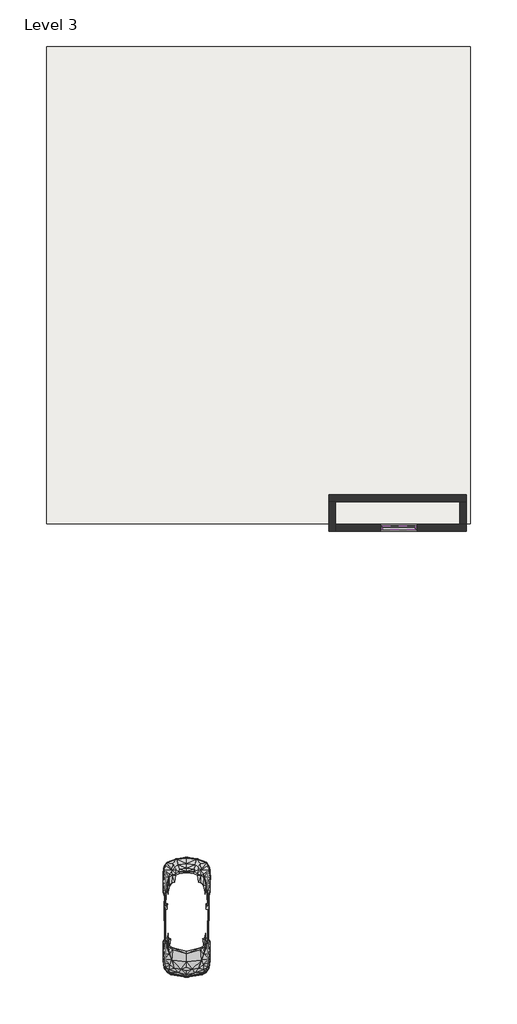
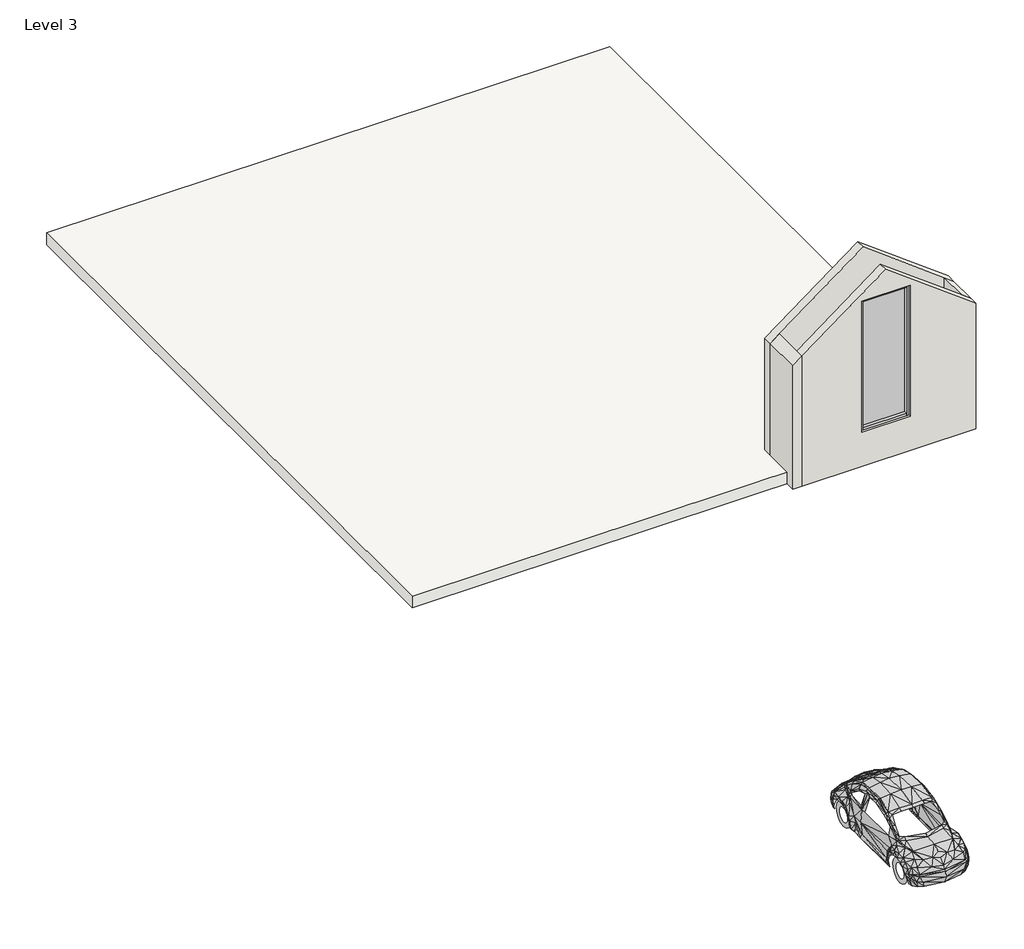
# One storey: 4 members, 4 walls, 1 plate, 1 proxy, 1 roof.
"""IFC4 building model written with IfcOpenShell, lengths in millimetres."""

from ifc_helpers import new_model, si_unit, frame, origin, place, context, project, spatial, polyline, outline, extrude, faceted_brep, transform, mapped, element, save
from components import rpc_beetle_rpc_beetle_31f8b51e, member_273a15f2, member_fce16bad, system_panel_glazed_8a71b067

model = new_model("IFC4")

# Units and contexts
model_context = context("Model", 3, world=origin())
ifc_project = project(units=[si_unit("LENGTHUNIT", "METRE", prefix="MILLI")], contexts=[model_context])

# Site, building, storey
site = spatial("IfcSite", under=ifc_project)
building = spatial("IfcBuilding", under=site)
storey = spatial("IfcBuildingStorey", under=building, Name="Level 3", Elevation=6096.0)

# Proxy
placement = place(None, origin())
rpc_beetle_rpc_beetle_shape = rpc_beetle_rpc_beetle_31f8b51e(model_context)
element("IfcBuildingElementProxy", 1, Name="RPC Beetle : RPC Beetle", ObjectType="RPC Beetle : RPC Beetle", at=placement, inside=storey, context=model_context, shape_type="MappedRepresentation", body=[
    mapped(rpc_beetle_rpc_beetle_shape, transform((-17203.6097681, -26062.0454888, 6096.0), x_axis=(-1.0, 0.0, 0.0), y_axis=(0.0, -1.0, 0.0), z_axis=(0.0, 0.0, 1.0))),
])

# Members
member_shape = member_273a15f2(model_context)
element("IfcMember", 2, ObjectType="Rectangular Mullion : 2.5\" x 5\" rectangular", at=placement, inside=storey, context=model_context, shape_type="MappedRepresentation", body=[
    mapped(member_shape, transform((-9620.2916763, -14382.9531473, 10458.2918565), x_axis=(0.0, 0.0, 1.0), y_axis=(0.0, -1.0, 0.0), z_axis=(1.0, 0.0, 0.0))),
])
element("IfcMember", 3, ObjectType="Rectangular Mullion : 2.5\" x 5\" rectangular", at=placement, inside=storey, context=model_context, shape_type="MappedRepresentation", body=[
    mapped(member_shape, transform((-10712.4916763, -14382.9531473, 7004.2917405), x_axis=(0.0, 0.0, -1.0), y_axis=(0.0, -1.0, 0.0), z_axis=(-1.0, 0.0, 0.0))),
])
member_2_shape = member_fce16bad(model_context)
element("IfcMember", 4, ObjectType="Rectangular Mullion : 2.5\" x 5\" rectangular", at=placement, inside=storey, context=model_context, shape_type="MappedRepresentation", body=[
    mapped(member_2_shape, transform((-9556.7916763, -14382.9531473, 7004.2917405), x_axis=(1.0, 0.0, 0.0), y_axis=(0.0, -1.0, 0.0), z_axis=(0.0, 0.0, -1.0))),
])
element("IfcMember", 5, ObjectType="Rectangular Mullion : 2.5\" x 5\" rectangular", at=placement, inside=storey, context=model_context, shape_type="MappedRepresentation", body=[
    mapped(member_2_shape, transform((-10775.9916763, -14382.9531473, 10458.2918565), x_axis=(-1.0, 0.0, 0.0), y_axis=(0.0, -1.0, 0.0), z_axis=(0.0, 0.0, 1.0))),
])

# Plate
system_panel_glazed_shape = system_panel_glazed_8a71b067(model_context)
element("IfcPlate", 6, ObjectType="System Panel : Glazed", at=placement, inside=storey, context=model_context, shape_type="MappedRepresentation", body=[
    mapped(system_panel_glazed_shape, transform((-10166.3916763, -14382.9531473, 7067.7917405), x_axis=(1.0, 0.0, 0.0), y_axis=(0.0, 1.0, 0.0), z_axis=(0.0, 0.0, 1.0))),
])

# Roof
element("IfcRoof", 7, ObjectType="Generic - 12\"", at=placement, inside=storey, context=model_context, shape_type="SweptSolid", body=[
    extrude(outline(polyline([(-21851.8097681, 1564.7660078), (-7792.9097681, 1564.7660078), (-7792.9097681, -14246.7339922), (-21851.8097681, -14246.7339922), (-21851.8097681, 1564.7660078)])), frame((0.0, 0.0, 6096.0), z_axis=(0.0, 0.0, 1.0), x_axis=(1.0, 0.0, 0.0)), (0.0, 0.0, 1.0), 304.8),
])

# Walls
element("IfcWall", 8, ObjectType="9\"", at=placement, inside=storey, context=model_context, shape_type="Brep", body=[
    faceted_brep([(-7918.4916763, -13290.7531473, 6096.0), (-12490.4916763, -13290.7531473, 6096.0), (-12490.4916763, -13290.7531473, 9352.9783777), (-10171.6547833, -13290.7531473, 11092.1060475), (-7918.4916763, -13290.7531473, 9402.2337173), (-7918.4916763, -13519.3531473, 6096.0), (-7918.4916763, -13519.3531473, 9402.2337173), (-8147.0916763, -13519.3531473, 9573.6837173), (-10171.6547833, -13519.3531473, 11092.1060475), (-12261.8916763, -13519.3531473, 9524.4283777), (-12490.4916763, -13519.3531473, 9352.9783777), (-12490.4916763, -13519.3531473, 6096.0), (-12261.8916763, -13519.3531473, 6096.0), (-8147.0916763, -13519.3531473, 6096.0)], [[[0, 1, 2, 3, 4]], [[5, 6, 7, 8, 9, 10, 11, 12, 13]], [[1, 0, 5, 13, 12, 11]], [[2, 1, 11, 10]], [[0, 4, 6, 5]], [[4, 3, 8, 7, 6]], [[3, 2, 10, 9, 8]]]),
])
element("IfcWall", 9, ObjectType="9\"", at=placement, inside=storey, context=model_context, shape_type="Brep", body=[
    faceted_brep([(-12490.4916763, -13519.3531473, 6096.0), (-12490.4916763, -14497.2531473, 6096.0), (-12490.4916763, -14497.2531473, 9352.9783777), (-12490.4916763, -13519.3531473, 9352.9783777), (-12261.8916763, -13519.3531473, 6096.0), (-12261.8916763, -13519.3531473, 9524.4283777), (-12261.8916763, -14268.6531473, 9524.4283777), (-12261.8916763, -14497.2531473, 9524.4283777), (-12261.8916763, -14497.2531473, 6096.0), (-12261.8916763, -14268.6531473, 6096.0)], [[[0, 1, 2, 3]], [[4, 5, 6, 7, 8, 9]], [[1, 0, 4, 9, 8]], [[0, 3, 5, 4]], [[2, 1, 8, 7]], [[3, 2, 7, 6, 5]]]),
])
element("IfcWall", 10, ObjectType="9\"", at=placement, inside=storey, context=model_context, shape_type="Brep", body=[
    faceted_brep([(-12261.8916763, -14497.2531473, 6096.0), (-7918.4916763, -14497.2531473, 6096.0), (-7918.4916763, -14497.2531473, 9402.2337173), (-10171.6547833, -14497.2531473, 11092.1060475), (-12261.8916763, -14497.2531473, 9524.4283777), (-10775.9916763, -14497.2531473, 7004.2917405), (-10775.9916763, -14497.2531473, 10458.2918565), (-9556.7916763, -14497.2531473, 10458.2918565), (-9556.7916763, -14497.2531473, 7004.2917405), (-7918.4916763, -14268.6531473, 6096.0), (-8147.0916763, -14268.6531473, 6096.0), (-12261.8916763, -14268.6531473, 6096.0), (-12261.8916763, -14268.6531473, 9524.4283777), (-10171.6547833, -14268.6531473, 11092.1060475), (-8147.0916763, -14268.6531473, 9573.6837173), (-7918.4916763, -14268.6531473, 9402.2337173), (-10775.9916763, -14268.6531473, 10458.2918565), (-10775.9916763, -14268.6531473, 7004.2917405), (-9556.7916763, -14268.6531473, 7004.2917405), (-9556.7916763, -14268.6531473, 10458.2918565)], [[[0, 1, 2, 3, 4], [5, 6, 7, 8]], [[9, 10, 11, 12, 13, 14, 15], [16, 17, 18, 19]], [[1, 0, 11, 10, 9]], [[0, 4, 12, 11]], [[2, 1, 9, 15]], [[12, 4, 3, 13]], [[2, 15, 14, 13, 3]], [[5, 17, 16, 6]], [[6, 16, 19, 7]], [[7, 19, 18, 8]], [[17, 5, 8, 18]]]),
])
element("IfcWall", 11, ObjectType="9\"", at=placement, inside=storey, context=model_context, shape_type="SweptSolid", body=[
    extrude(outline(polyline([(6096.0, -7918.4916763), (9402.2337173, -7918.4916763), (9573.6837173, -8147.0916763), (6096.0, -8147.0916763), (6096.0, -7918.4916763)])), frame((0.0, -14268.6531473, 0.0), z_axis=(0.0, 1.0, 0.0), x_axis=(0.0, 0.0, 1.0)), (0.0, 0.0, 1.0), 749.3),
])

save(model, "model.ifc")

# Revit data of these elements
# Type "RPC Beetle : RPC Beetle"
#   built-in parameter 1005198 = "{2, 15},{39, RPC-16-0U6E-L4EG-ENH1-J3KF-SVEL-0TX4-C0},{1, 0},{1, 0},{2, 36},{1, 8},{5, Color},{1, 0},{1, 0},{3, 0.8},{3, 0.8},{3, 0.8},{1, 8},{7, BBoxMin},{1, 0},{1, 0},{1, 0},{1, 0},{1, 0},{1, 8},{7, BBoxMax},{1, 0},{1, 0},{1, 0},{1, 0},{1, 0},{2, 11},{9, RPCTypeId},{1, 0},{1, 0},{39, RPC-16-0U6E-L4EG-ENH1-J3KF-SVEL-0TX4-C0},{1, 6},{14, RPCPlantHeight},{1, 0},{1, 0},{7, 4.91667},{2, 11},{20, AdvancedUIDefinition},{1, 0},{1, 0},{0, },{2, 11},{10, AssetLibID},{1, 0},{1, 0},{36, 4D3F6E72-3F99-4203-98E9-AF80B3C7A7A4},{2, 11},{10, BaseSchema},{1, 0},{1, 0},{9, RPCSchema},{2, 11},{12, ExchangeGUID},{1, 0},{1, 0},{0, },{1, 2},{6, Hidden},{1, 0},{1, 0},{1, 0},{2, 11},{12, LocalizedUID},{1, 0},{1, 0},{0, },{1, 4},{11, RPCCategory},{1, 0},{1, 0},{1, 0},{2, 11},{8, RPCImage},{1, 0},{1, 0},{0, },{1, 4},{13, SchemaVersion},{1, 0},{1, 0},{1, 4},{2, 11},{12, UIDefinition},{1, 0},{1, 0},{0, },{2, 11},{6, UIName},{1, 0},{1, 0},{39, RPC-16-0U6E-L4EG-ENH1-J3KF-SVEL-0TX4-C0},{2, 11},{11, VersionGUID},{1, 0},{1, 0},{9, RPCSchema},{2, 11},{9, assettype},{1, 0},{1, 0},{11, RPCGeometry},{2, 11},{11, description},{1, 0},{1, 0},{0, },{2, 11},{9, localname},{1, 0},{1, 0},{3, RPC},{2, 11},{9, localtype},{1, 0},{1, 0},{3, RPC},{1, 4},{8, revision},{1, 0},{1, 0},{1, 1},{2, 11},{9, thumbnail},{1, 0},{1, 0},{0, },{1, 4},{7, version},{1, 0},{1, 0},{1, 1},{2, 14},{6, Height},{1, 0},{1, 0},{7, 4.91667},{1, 2},{20, RPC_Cast Reflections},{1, 0},{1, 0},{1, 1},{1, 4},{16, RPC_Transparency},{1, 0},{1, 0},{2, 18},{1, 4},{11, RPC_Tinting},{1, 0},{1, 0},{2, 50},{1, 2},{15, RPC_Use Tinting},{1, 0},{1, 0},{1, 0},{1, 2},{17, RPC_License Plate},{1, 0},{1, 0},{1, 0},{2, 11},{25, RPC_License Plate Texture},{1, 0},{1, 0},{64, __RPC:/object data/textures/car/plate/textures/default/rgb/0/0/0},{2, 11},{27, RPC_i_License Plate Texture},{1, 0},{1, 0},{0, },{1, 2},{16, RPC_Custom Plate},{1, 0},{1, 0},{1, 0},{2, 11},{27, RPC_License Plate File Name},{1, 0},{1, 0},{0, },{2, 11},{7, keyword},{1, 0},{1, 0},{27, :Geometry:RPC:VW Beetle [4]},{2, 11},{8, category},{1, 0},{1, 0},{21, :Auto_Economy/Midsize},{21, assetlibrary_base.fbx},{1, 5},"
#   built-in parameter 1005195 = "RPC-16-0U6E-L4EG-ENH1-J3KF-SVEL-0TX4-C0"
#   Height = 0
# Type "Rectangular Mullion : 2.5\" x 5\" rectangular"
#   built-in parameter 1007304 = 0.416667 (stored number, unit not read)
#   built-in parameter 1007301 = 0.104167 (stored number, unit not read)
#   built-in parameter 1007300 = 0.104167 (stored number, unit not read)
# Type "System Panel : Glazed"
#   Construction Type Id = "GSP4R"
#   Analytic Construction = "1/8 in Pilkington single glazing"
#   Visual Light Transmittance = 0.9
#   Solar Heat Gain Coefficient = 0.86
#   Heat Transfer Coefficient (U) = 1.18115 BTU/(h·ft²·°F)
#   Define Thermal Properties by = 1
# Type "Generic - 12\""
#   Assembly Code = "B1020"
#   Layers, outside or top first: 1' - 0" no material (function 1)
# Type "9\""
#   Assembly Code = "B2010"
#   Layers, outside or top first: 0' - 9" no material (function 1)
# Element 1 (IfcBuildingElementProxy, "RPC Beetle : RPC Beetle")
#   Phase Created = New Construction
# Elements 2, 3, 4, 5 (IfcMember, "Rectangular Mullion : 2.5\" x 5\" rectangular")
#   Phase Created = New Construction
#   Materials on its faces: "Aluminum"
# Element 6 (IfcPlate, "System Panel : Glazed")
#   Phase Created = New Construction
#   Materials on its faces: "Glass"
# Element 7 (IfcRoof, "Generic - 12\"")
#   built-in parameter 1001705 = 21 (stored number, unit not read)
#   built-in parameter 1001710 = 33615
#   Phase Created = New Construction
#   Materials on its faces: "Default Roof"
# Elements 8, 9, 10, 11 (IfcWall, "9\"")
#   Top Offset = 0' - 0"
#   Base Offset = 0' - 0"
#   Unconnected Height = 10' - 0"
#   wall height = 10' - 0"
#   Phase Created = New Construction
#   Base Constraint = Level 3
#   Materials on its faces: "Default Wall"
# Materials
#   "Aluminum": class "Metal", colour RGB 247 247 247, transparency 0, Description = "Aluminum 6061", Cost = 0
#   "Glass": class "Glass", colour RGB 0 128 192, transparency 0.75, Description = "Soda Lime Glass", Cost = 0
#   "Default Roof": colour RGB 88 101 114, transparency 0, Cost = 0
#   "Default Wall": colour RGB 128 128 128, transparency 0, Cost = 0
